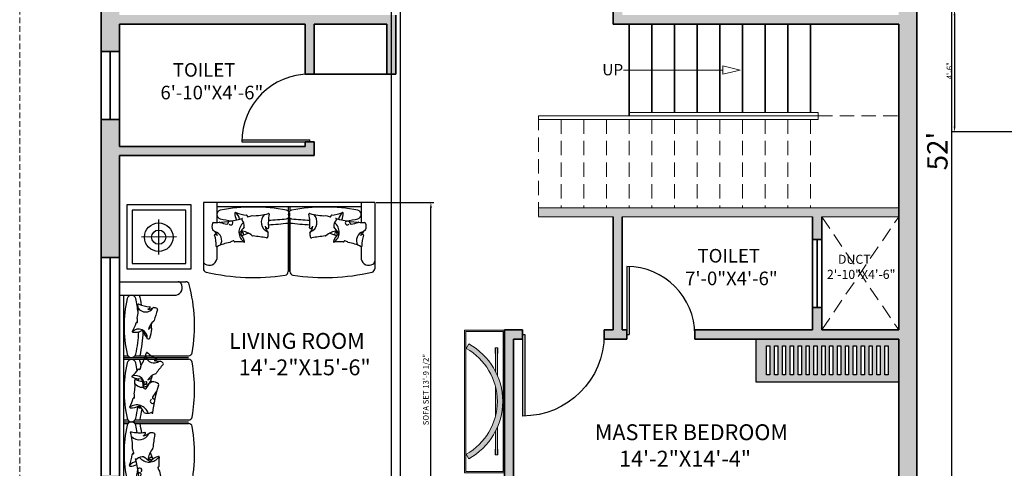
# Model space of a CAD drawing. Units: inches. Extents: x 1566 to 2546, y 1087 to 2705.
# Tile 6 of 27: x 1606 to 2040, y 1326 to 1524. Entities that reach past the tile are written whole.
import ezdxf

# ---------------------------------------------------------------- set-up
doc = ezdxf.new("R2010")
doc.units = ezdxf.units.IN
doc.linetypes.add('DASHED', pattern=[19.05, 12.7, -6.35])
for name, color, linetype, lineweight in [('A-ANNO-DIMS', 2, 'Continuous', 18), ('A-ANNO-TEXT', 7, 'Continuous', 18), ('A-AREA-IDEN', 7, 'Continuous', 18), ('A-DOOR', 4, 'Continuous', 25), ('A-FLOR-OVHD', 8, 'DASHED', 18), ('A-FLOR-STRS', 3, 'Continuous', 18), ('A-FURN', 8, 'Continuous', 18), ('A-WALL', 7, 'Continuous', 35), ('A-WALL-PATT', 8, 'Continuous', 13), ('aparador', 36, 'Continuous', 9), ('moveis', 254, 'Continuous', 5)]:
    doc.layers.add(name, color=color, linetype=linetype, lineweight=lineweight)
for name, color, linetype in [('HID', 11, 'Continuous'), ('MESA', 7, 'Continuous'), ('SAN', 5, 'Continuous'), ('wood', 26, 'Continuous')]:
    doc.layers.add(name, color=color, linetype=linetype)
doc.styles.get("Standard").update_dxf_attribs({"font": 'arial.ttf'})
doc.dimstyles.new('ISO-25', dxfattribs={"dimtxt": 2.5, "dimasz": 2.5, "dimexe": 1.25, "dimexo": 0.625, "dimtad": 1, "dimtxsty": 'Standard', "dimcen": 2.5, "dimadec": 0, "dimazin": 0, "dimtfac": 1, "dimtmove": 0, "dimatfit": 3, "dimfxl": 1, "dimarcsym": 0})

# ---------------------------------------------------------------- blocks, each defined once
blk = doc.blocks.new('d2')
for p, q in [((3364.08, 1632.29), (3364.08, 1602.29)), ((3365.08, 1632.29), (3365.08, 1602.29)), ((3364.08, 1602.29), (3365.08, 1602.29))]:
    blk.add_line(p, q)
at = {"ltscale": 0.3}
blk.add_arc((3364.08, 1602.29), 30, 0, 90, dxfattribs=at)
blk = doc.blocks.new('d1')
for p, q in [((3297.32, 1596.93), (3297.32, 1632.93)), ((3298.32, 1596.93), (3298.32, 1632.93)), ((3297.32, 1596.93), (3298.32, 1596.93))]:
    blk.add_line(p, q)
at = {"ltscale": 0.3}
blk.add_arc((3297.32, 1596.93), 36, 0, 90, dxfattribs=at)
blk = doc.blocks.new('*D7')
at = {"layer": 'A-ANNO-DIMS', "color": 0, "lineweight": -2, "transparency": 16777216}
for p, q in [((2002.15, 1778.2), (2018.24, 1778.2)), ((2016.99, 1156.7), (2016.99, 1775.7)), ((2002.15, 1154.2), (2018.24, 1154.2))]:
    blk.add_line(p, q, dxfattribs=at)
at = {"layer": 'A-ANNO-DIMS', "color": 0, "transparency": 16777216}
for points in [[(2016.58, 1775.7), (2017.41, 1775.7), (2016.99, 1778.2)], [(2016.58, 1156.7), (2017.41, 1156.7), (2016.99, 1154.2)]]:
    blk.add_solid(points, dxfattribs=at)
at = {"layer": 'Defpoints', "color": 0, "transparency": 16777216}
for p in [(2001.53, 1778.2), (2016.99, 1778.2), (2001.53, 1154.2)]:
    blk.add_point(p, dxfattribs=at)
at = {"layer": 'A-ANNO-DIMS', "color": 0, "transparency": 16777216, "insert": (2011.77, 1466.2), "char_height": 9, "attachment_point": 5, "rotation": 90}
blk.add_mtext("52'", dxfattribs=at)
blk = doc.blocks.new('Banco Lintz')
at = {"layer": 'MESA', "ltscale": 0.05}
h = blk.add_hatch(color=256, dxfattribs=at)
h.dxf.hatch_style = 1
h.set_gradient(color1=(138, 84, 66), color2=(0, 0, 0), one_color=1, name='INVCYLINDER')
h.paths.add_polyline_path([(0.48, 0), (0, 0), (0, -1.6), (0.48, -1.6)])
h.paths.add_polyline_path([(0.403, -0.509), (0.077, -0.509), (0.077, -0.472), (0.403, -0.472)], flags=16)
h.paths.add_polyline_path([(0.403, -0.561), (0.403, -0.597), (0.077, -0.597), (0.077, -0.561)], flags=16)
h.paths.add_polyline_path([(0.403, -0.421), (0.077, -0.421), (0.077, -0.384), (0.403, -0.384)], flags=16)
h.paths.add_polyline_path([(0.403, -0.649), (0.403, -0.686), (0.077, -0.686), (0.077, -0.649)], flags=16)
h.paths.add_polyline_path([(0.403, -0.332), (0.077, -0.332), (0.077, -0.296), (0.403, -0.296)], flags=16)
h.paths.add_polyline_path([(0.403, -0.737), (0.403, -0.774), (0.077, -0.774), (0.077, -0.737)], flags=16)
h.paths.add_polyline_path([(0.403, -0.244), (0.077, -0.244), (0.077, -0.207), (0.403, -0.207)], flags=16)
h.paths.add_polyline_path([(0.403, -0.826), (0.403, -0.863), (0.077, -0.863), (0.077, -0.826)], flags=16)
h.paths.add_polyline_path([(0.403, -0.156), (0.077, -0.156), (0.077, -0.119), (0.403, -0.119)], flags=16)
h.paths.add_polyline_path([(0.403, -0.914), (0.403, -0.951), (0.077, -0.951), (0.077, -0.914)], flags=16)
h.paths.add_polyline_path([(0.403, -1.003), (0.403, -1.039), (0.077, -1.039), (0.077, -1.003)], flags=16)
h.paths.add_polyline_path([(0.403, -1.091), (0.403, -1.128), (0.077, -1.128), (0.077, -1.091)], flags=16)
h.paths.add_polyline_path([(0.403, -1.179), (0.403, -1.216), (0.077, -1.216), (0.077, -1.179)], flags=16)
h.paths.add_polyline_path([(0.403, -1.268), (0.403, -1.304), (0.077, -1.304), (0.077, -1.268)], flags=16)
h.paths.add_polyline_path([(0.403, -1.356), (0.403, -1.393), (0.077, -1.393), (0.077, -1.356)], flags=16)
h.paths.add_polyline_path([(0.403, -1.444), (0.403, -1.481), (0.077, -1.481), (0.077, -1.444)], flags=16)
for points in [[(0, -1.6), (0.48, -1.6), (0.48, 0), (0, 0)], [(0.077, -0.119), (0.403, -0.119), (0.403, -0.156), (0.077, -0.156)], [(0.077, -0.207), (0.403, -0.207), (0.403, -0.244), (0.077, -0.244)], [(0.077, -0.296), (0.403, -0.296), (0.403, -0.332), (0.077, -0.332)], [(0.077, -0.384), (0.403, -0.384), (0.403, -0.421), (0.077, -0.421)], [(0.077, -0.472), (0.403, -0.472), (0.403, -0.509), (0.077, -0.509)], [(0.077, -0.561), (0.403, -0.561), (0.403, -0.597), (0.077, -0.597)], [(0.077, -0.649), (0.403, -0.649), (0.403, -0.686), (0.077, -0.686)], [(0.077, -0.737), (0.403, -0.737), (0.403, -0.774), (0.077, -0.774)], [(0.077, -0.826), (0.403, -0.826), (0.403, -0.863), (0.077, -0.863)], [(0.077, -0.914), (0.403, -0.914), (0.403, -0.951), (0.077, -0.951)], [(0.077, -1.003), (0.403, -1.003), (0.403, -1.039), (0.077, -1.039)], [(0.077, -1.091), (0.403, -1.091), (0.403, -1.128), (0.077, -1.128)], [(0.077, -1.179), (0.403, -1.179), (0.403, -1.216), (0.077, -1.216)], [(0.077, -1.268), (0.403, -1.268), (0.403, -1.304), (0.077, -1.304)], [(0.077, -1.356), (0.403, -1.356), (0.403, -1.393), (0.077, -1.393)], [(0.077, -1.444), (0.403, -1.444), (0.403, -1.481), (0.077, -1.481)]]:
    blk.add_lwpolyline(points, close=True, dxfattribs=at)
blk = doc.blocks.new('Aparador ORGANICA Formatto')
at = {"layer": 'aparador', "ltscale": 0.3}
h = blk.add_hatch(color=256, dxfattribs=at)
h.dxf.hatch_style = 1
h.set_gradient(color1=(118, 213, 123), color2=(52, 168, 57), one_color=1, tint=0.43, name='INVCURVED')
h.paths.add_polyline_path([(0.8, 0.45), (-0.8, 0.45), (-0.8, 0), (0.8, 0)])
h.paths.add_polyline_path([(0.785, 0.435), (0.785, 0.015), (-0.785, 0.015), (-0.785, 0.435)], flags=16)
h.paths.add_polyline_path([(0.291, 0.37), (0.537, 0.37), (0.537, 0.376), (0.601, 0.376), (0.601, 0.37), (0.601, 0.35), (0.601, 0.344), (0.537, 0.344), (0.537, 0.35), (0.334, 0.35, -0.150336), (0.645, 0.049), (0.592, 0.02, 0.208852), (0.163, 0.35), (-0.163, 0.35, 0.208852), (-0.592, 0.02), (-0.645, 0.049, -0.150336), (-0.334, 0.35), (-0.537, 0.35), (-0.537, 0.344), (-0.601, 0.344), (-0.601, 0.35), (-0.601, 0.37), (-0.601, 0.376), (-0.537, 0.376), (-0.537, 0.37), (-0.291, 0.37, -0.206106)], flags=0)
h = blk.add_hatch(color=256, dxfattribs=at)
h.dxf.hatch_style = 1
h.set_gradient(color1=(135, 92, 69), color2=(0, 0, 0), one_color=1, name='INVCURVED')
h.paths.add_polyline_path([(-0.645, 0.049), (-0.592, 0.02, -0.590888), (0.592, 0.02), (0.645, 0.049, 0.590888)])
h = blk.add_hatch(color=256, dxfattribs=at)
h.dxf.hatch_style = 1
h.set_gradient(color1=(178, 189, 189), one_color=1, tint=1, name='CYLINDER')
h.paths.add_polyline_path([(-0.537, 0.376), (-0.601, 0.376), (-0.601, 0.37), (-0.537, 0.37)])
h.paths.add_polyline_path([(-0.537, 0.35), (-0.601, 0.35), (-0.601, 0.344), (-0.537, 0.344)])
h = blk.add_hatch(color=256, dxfattribs=at)
h.dxf.hatch_style = 1
h.set_gradient(color1=(118, 213, 123), color2=(31, 101, 35), one_color=1, tint=0.26, name='INVCURVED')
h.paths.add_polyline_path([(-0.291, 0.37), (-0.601, 0.37), (-0.601, 0.35), (-0.334, 0.35, -0.015999)])
h = blk.add_hatch(color=256, dxfattribs=at)
h.dxf.hatch_style = 1
h.set_gradient(color1=(118, 213, 123), color2=(31, 101, 35), one_color=1, tint=0.26, name='INVCURVED')
h.paths.add_polyline_path([(-0.163, 0.35), (0.163, 0.35, 0.122516)])
h = blk.add_hatch(color=256, dxfattribs=at)
h.dxf.hatch_style = 1
h.set_gradient(color1=(118, 213, 123), color2=(31, 101, 35), one_color=1, tint=0.26, name='INVCURVED')
h.paths.add_polyline_path([(0.601, 0.37), (0.291, 0.37, -0.015999), (0.334, 0.35), (0.601, 0.35)])
h = blk.add_hatch(color=256, dxfattribs=at)
h.dxf.hatch_style = 1
h.set_gradient(color1=(178, 189, 189), one_color=1, tint=1, name='CYLINDER')
h.paths.add_polyline_path([(0.601, 0.376), (0.537, 0.376), (0.537, 0.37), (0.601, 0.37)])
h.paths.add_polyline_path([(0.601, 0.35), (0.537, 0.35), (0.537, 0.344), (0.601, 0.344)])
for p, q in [((-0.592, 0.02), (-0.645, 0.049)), ((0.592, 0.02), (0.645, 0.049))]:
    blk.add_line(p, q, dxfattribs=at)
for points in [[(-0.601, 0.37), (-0.601, 0.376), (-0.537, 0.376), (-0.537, 0.37)], [(-0.537, 0.35), (-0.537, 0.344), (-0.601, 0.344), (-0.601, 0.35)], [(0.601, 0.37), (0.601, 0.376), (0.537, 0.376), (0.537, 0.37)], [(0.537, 0.35), (0.537, 0.344), (0.601, 0.344), (0.601, 0.35)]]:
    blk.add_lwpolyline(points, dxfattribs=at)
for radius in [0.736, 0.676]:
    blk.add_arc((0, -0.306), radius, 28.8434, 151.1566, dxfattribs=at)
at = {"layer": 'moveis', "ltscale": 0.3}
for p, q in [((-0.601, 0.37), (-0.601, 0.35)), ((-0.291, 0.37), (-0.601, 0.37)), ((-0.601, 0.35), (-0.334, 0.35)), ((-0.163, 0.35), (0.163, 0.35)), ((0.291, 0.37), (0.601, 0.37)), ((0.601, 0.35), (0.334, 0.35)), ((0.601, 0.37), (0.601, 0.35))]:
    blk.add_line(p, q, dxfattribs=at)
for points in [[(-0.8, 0), (0.8, 0), (0.8, 0.45), (-0.8, 0.45)], [(-0.785, 0.015), (0.785, 0.015), (0.785, 0.435), (-0.785, 0.435)]]:
    blk.add_lwpolyline(points, close=True, dxfattribs=at)
blk = doc.blocks.new('123')
at = {"layer": 'HID'}
for centre, radius, start, end in [((1246.02, 1434.08), 0.283, 70.5302, 181.6176), ((1243.23, 1430.56), 4.68, 10.8696, 54.3073), ((1254.03, 1456.71), 23.73, 250.5302, 262.522), ((1285.34, 1456.71), 23.73, 277.478, 289.4698), ((1296.13, 1430.56), 4.68, 125.6927, 169.1304), ((1293.34, 1434.08), 0.283, 358.3824, 109.4698), ((1236.34, 1429.49), 0.472, 90.5535, 158.334), ((1235.86, 1479.09), 49.13, 270.5535, 285.4148), ((1235.86, 1479.09), 49.13, 270.5535, 273.614), ((1238.99, 1429.59), 0.472, 66.2045, 93.614), ((1245.71, 1450.89), 21.87, 252.6177, 260.951), ((1243.86, 1429.85), 1.05, 142.8444, 177.2985), ((1243.29, 1429.88), 0.472, 177.2985, 187.3574), ((1243.92, 1429.87), 0.999, 224.2238, 57.6435), ((1253.29, 1434.28), 7.55, 181.6176, 204.8398), ((1252.86, 1425.7), 5.32, 127.6048, 236.1053), ((1249.25, 1431.33), 0.472, 105.6578, 222.8337), ((1246.1, 1428.4), 3.83, 354.2387, 42.8337), ((1250.9, 1432.91), 0.283, 348.0525, 82.522), ((1251.46, 1432.79), 0.283, 168.0525, 279.4331), ((1249.65, 1443.68), 11.32, 279.4331, 289.3248), ((1254.03, 1456.71), 23.73, 268.4714, 286.0168), ((1262.09, 1430.12), 4.71, 134.8494, 245.9788), ((1279.38, 1429.58), 18.88, 167.7826, 186.0053), ((1260.65, 1433.64), 0.283, 347.7826, 106.0168), ((1278.71, 1433.64), 0.283, 73.9832, 192.2174), ((1259.98, 1429.58), 18.88, 353.9947, 12.2174), ((1285.34, 1456.71), 23.73, 253.9832, 271.5286), ((1277.28, 1430.12), 4.71, 294.0212, 45.1506), ((1289.72, 1443.68), 11.32, 250.6752, 260.5669), ((1287.91, 1432.79), 0.283, 260.5669, 11.9475), ((1288.46, 1432.91), 0.283, 97.478, 191.9475), ((1293.27, 1428.4), 3.83, 137.1663, 185.7613), ((1286.5, 1425.7), 5.32, 303.8947, 52.3952), ((1290.11, 1431.33), 0.472, 317.1663, 74.3422), ((1303.5, 1479.09), 49.13, 254.5852, 269.4465), ((1286.07, 1434.28), 7.55, 335.1602, 358.3824), ((1295.45, 1429.87), 0.999, 122.3565, 315.7762), ((1295.5, 1429.85), 1.05, 2.7015, 37.1556), ((1296.08, 1429.88), 0.472, 352.6426, 2.7015), ((1293.65, 1450.89), 21.87, 279.049, 287.3823), ((1300.38, 1429.59), 0.472, 86.386, 113.7955), ((1303.5, 1479.09), 49.13, 266.386, 269.4465), ((1303.02, 1429.49), 0.472, 21.666, 89.4465), ((1239.48, 1428.24), 3.85, 158.334, 202.6623), ((1236.36, 1426.94), 0.472, 202.6623, 238.3929), ((1233.54, 1422.36), 4.91, 20.2155, 58.3929), ((1236.02, 1422.11), 3.93, 326.1078, 77.2372), ((1242.35, 1429.76), 0.472, 260.951, 7.3574), ((1285.54, 1398.1), 46.53, 139.9755, 144.1671), ((1247.81, 1425.22), 0.945, 310.8427, 57.338), ((1253.61, 1432.21), 7.94, 229.38, 238.0577), ((1248.02, 1418.03), 8.16, 48.6039, 87.0681), ((1260.85, 1429.07), 1.87, 202.9525, 250.443), ((1264.95, 1429.26), 5.89, 188.9571, 220.4913), ((1260.32, 1427.58), 0.283, 250.443, 6.0053), ((1279.04, 1427.58), 0.283, 173.9947, 289.557), ((1274.42, 1429.26), 5.89, 319.5087, 351.0429), ((1278.51, 1429.07), 1.87, 289.557, 337.0475), ((1291.34, 1418.03), 8.16, 92.9319, 131.3961), ((1253.83, 1398.1), 46.53, 35.8329, 40.0245), ((1285.75, 1432.21), 7.94, 301.9423, 310.62), ((1291.56, 1425.22), 0.945, 122.662, 229.1573), ((1297.02, 1429.76), 0.472, 172.6426, 279.049), ((1303.34, 1422.11), 3.93, 102.7628, 213.8922), ((1305.82, 1422.36), 4.91, 121.6071, 159.7845), ((1303, 1426.94), 0.472, 301.6071, 337.3377), ((1299.88, 1428.24), 3.85, 337.3377, 21.666), ((1237.05, 1424.48), 0.236, 81.7015, 197.2637), ((1221.8, 1419.74), 15.74, 359.041, 17.2637), ((1236.86, 1423.18), 1.56, 34.2109, 81.7015), ((1248.4, 1413.06), 9.43, 110.6915, 120.5832), ((1245.15, 1421.66), 0.236, 359.311, 110.6915), ((1245.62, 1421.66), 0.236, 179.311, 273.7804), ((1246.94, 1401.69), 19.77, 81.7886, 93.7804), ((1248.01, 1425.2), 0.236, 144.1671, 251.1685), ((1243.89, 1420.15), 6.29, 12.876, 50.0789), ((1227.67, 1473.6), 52.85, 292.7112, 293.5018), ((1268.16, 1374.24), 53.54, 107.709, 111.2519), ((1248.79, 1424.95), 0.814, 313.9174, 40.1627), ((1249.8, 1421.5), 0.236, 261.7886, 12.876), ((1249.8, 1421.5), 0.236, 261.7886, 12.876), ((1253.8, 1424.57), 0.567, 227.5655, 264.8479), ((1248.46, 1365.29), 58.96, 79.0518, 84.8479), ((1259.76, 1423.73), 0.567, 259.0518, 342.8696), ((1256.05, 1424.88), 4.45, 342.8696, 7.2038), ((1283.31, 1424.88), 4.45, 172.7962, 197.1304), ((1279.6, 1423.73), 0.567, 197.1304, 280.9482), ((1290.9, 1365.29), 58.96, 95.1521, 100.9482), ((1285.56, 1424.57), 0.567, 275.1521, 312.4345), ((1271.2, 1374.24), 53.54, 68.7481, 72.291), ((1289.57, 1421.5), 0.236, 167.124, 278.2114), ((1289.57, 1421.5), 0.236, 167.124, 278.2114), ((1295.47, 1420.15), 6.29, 129.9211, 167.124), ((1292.43, 1401.69), 19.77, 86.2196, 98.2114), ((1290.58, 1424.95), 0.814, 139.8373, 226.0826), ((1311.69, 1473.6), 52.85, 246.4982, 247.2888), ((1291.36, 1425.2), 0.236, 288.8315, 35.8329), ((1293.75, 1421.66), 0.236, 266.2196, 0.689), ((1294.22, 1421.66), 0.236, 69.3085, 180.689), ((1290.97, 1413.06), 9.43, 59.4168, 69.3085), ((1302.5, 1423.18), 1.56, 98.2985, 145.7891), ((1317.56, 1419.74), 15.74, 162.7363, 180.959), ((1302.31, 1424.48), 0.236, 342.7363, 98.2985), ((1237.77, 1419.48), 0.236, 179.041, 297.2752), ((1246.94, 1401.69), 19.77, 99.7298, 117.2752), ((1292.43, 1401.69), 19.77, 62.7248, 80.2702), ((1301.6, 1419.48), 0.236, 242.7248, 0.959), ((1183.3, 1391.63), 19.77, 348.4714, 6.0168), ((1203.2, 1393.73), 0.236, 67.7826, 186.0168), ((1206.29, 1394.4), 3.93, 214.8494, 325.9788), ((1209.24, 1408.51), 15.74, 247.7826, 266.0053), ((1206.97, 1393.23), 1.56, 282.9525, 330.443), ((1207.41, 1396.62), 4.91, 268.9571, 300.4913), ((1208.12, 1392.58), 0.236, 330.443, 86.0053), ((1209.72, 1388.68), 3.71, 62.8696, 87.2038), ((1257.53, 1373.83), 49.13, 159.0518, 164.8479), ((1211.2, 1391.57), 0.472, 339.0518, 62.8696), ((1193.36, 1386.15), 9.43, 359.4331, 9.3248), ((1209.64, 1386.8), 0.472, 307.5655, 344.8479), ((1203.21, 1378.98), 3.9, 356.4825, 134.3073), ((1183.3, 1391.63), 19.77, 330.5302, 342.522), ((1201.6, 1387.78), 6.29, 261.6176, 299.5758), ((1202.38, 1385.62), 0.236, 68.0525, 162.522), ((1202.56, 1386.06), 0.236, 248.0525, 359.4331), ((1204.83, 1382.1), 0.236, 32.8897, 119.5758), ((1165.95, 1356.96), 46.53, 28.8632, 32.8897), ((1213.67, 1381.56), 6.13, 127.5655, 169.079), ((1204.32, 1386.81), 5.27, 309.1869, 318.5341), ((1191.35, 1384.83), 17.84, 340.6607, 353.8744), ((1208.63, 1383.01), 0.472, 349.5475, 138.5341), ((1199.58, 1383.44), 9.43, 359.0692, 11.4619), ((1200.72, 1381.79), 0.236, 150.5302, 261.6176), ((1207.62, 1379.5), 0.917, 184.9476, 286.1991), ((1207.74, 1379.07), 0.472, 286.1991, 340.6607), ((1187.51, 1377.19), 19.77, 328.4714, 346.0168), ((1210.06, 1371.93), 3.93, 194.8494, 305.9788), ((1206.93, 1372.36), 0.236, 47.7826, 166.0168), ((1217.66, 1384.18), 15.74, 227.7826, 246.0053), ((1210.31, 1370.6), 1.56, 262.9525, 310.443), ((1211.88, 1373.63), 4.91, 248.9571, 280.4913), ((1211.17, 1369.59), 0.236, 310.443, 66.0053), ((1187.51, 1377.19), 19.77, 310.5302, 322.522), ((1203.39, 1365.02), 0.236, 48.0525, 142.522), ((1203.71, 1365.37), 0.236, 228.0525, 339.4331), ((1195.1, 1368.6), 9.43, 339.4331, 349.3248), ((1251.18, 1335.08), 49.13, 139.0518, 144.8479), ((1211.34, 1365.39), 3.71, 42.8696, 67.2038), ((1213.71, 1367.59), 0.472, 319.0518, 42.8696), ((1200.52, 1361.98), 0.236, 130.5302, 241.6176), ((1201.9, 1358.5), 3.9, 336.4825, 114.3073), ((1203.4, 1367.31), 6.29, 241.6176, 279.5758), ((1181.91, 1357.9), 19.77, 349.7298, 7.2752), ((1201.76, 1360.43), 0.236, 69.041, 187.2752), ((1207.47, 1375.34), 15.74, 249.041, 267.2637), ((1204.48, 1360.87), 0.236, 12.8897, 99.5758), ((1159.36, 1350.55), 46.53, 8.8632, 12.8897), ((1212.61, 1357.35), 6.13, 107.5655, 149.079), ((1205.62, 1365.47), 5.27, 289.1869, 298.5341), ((1208.36, 1360.43), 0.472, 329.5475, 118.5341), ((1200.01, 1363.93), 9.43, 339.0692, 351.4619), ((1210.62, 1363.64), 0.472, 287.5655, 324.8479), ((1204.83, 1361.17), 3.93, 216.1078, 327.2372), ((1206.22, 1357.48), 0.917, 164.9476, 266.1991), ((1205.91, 1363.41), 4.91, 270.2155, 308.3929), ((1205.54, 1360.02), 1.56, 284.2109, 331.7015), ((1206.19, 1357.03), 0.472, 266.1991, 320.6607), ((1192.75, 1368.04), 17.84, 320.6607, 333.8744), ((1206.71, 1359.39), 0.236, 331.7015, 87.2637), ((1209.25, 1359.2), 0.472, 92.6623, 128.3929), ((1209.41, 1355.82), 3.85, 48.334, 92.6623), ((1258.43, 1341.83), 49.13, 160.5535, 175.4148), ((1258.43, 1341.83), 49.13, 160.5535, 163.614), ((1211.66, 1358.35), 0.472, 340.5535, 48.334), ((1181.91, 1357.9), 19.77, 331.7886, 343.7804), ((1201.12, 1352.31), 0.236, 69.311, 163.7804), ((1201.29, 1352.75), 0.236, 249.311, 0.6915), ((1192.09, 1352.64), 9.43, 0.6915, 10.5832), ((1209.42, 1351.1), 0.999, 114.2238, 307.6435), ((1209.85, 1352.61), 0.472, 150.951, 257.3574), ((1228.56, 1342.22), 21.87, 142.6177, 150.951), ((1209.65, 1351.69), 0.472, 67.2985, 77.3574), ((1209.42, 1351.16), 1.05, 32.8444, 67.2985), ((1210.84, 1355.82), 0.472, 316.2045, 343.614), ((1202.44, 1344.12), 5.32, 17.6048, 126.1053), ((1199.54, 1348.44), 0.236, 151.7886, 262.876), ((1199.54, 1348.44), 0.236, 151.7886, 262.876), ((1200.29, 1354.45), 6.29, 262.876, 300.0789), ((1203.73, 1349.03), 0.945, 200.8427, 307.338), ((1256.07, 1351.41), 52.85, 182.7112, 183.5018), ((1203.63, 1348.85), 0.236, 34.1671, 141.1685), ((1165.33, 1322.86), 46.53, 29.9755, 34.1671), ((1155.85, 1369.08), 52.85, 337.2794, 337.2982), ((1207.3, 1349.55), 3.83, 244.2387, 292.8337), ((1208.97, 1345.59), 0.472, 355.6578, 112.8337), ((1199.97, 1337.3), 0.283, 77.7826, 196.0168), ((1176.89, 1330.67), 23.73, 358.4714, 16.0168), ((1204.03, 1356.03), 18.88, 257.7826, 276.0053), ((1203.48, 1338.74), 4.71, 224.8494, 335.9788), ((1204.35, 1341.6), 5.89, 278.9571, 310.4913), ((1204.54, 1337.5), 1.87, 292.9525, 340.443), ((1206.03, 1336.97), 0.283, 340.443, 96.0053), ((1208.73, 1332.7), 4.45, 72.8696, 97.2038), ((1268.32, 1325.11), 58.96, 169.0518, 174.8479), ((1209.88, 1336.41), 0.567, 349.0518, 72.8696), ((1189.93, 1326.3), 11.32, 9.4331, 19.3248), ((1215.58, 1324.67), 8.16, 138.6039, 177.0681), ((1209.03, 1330.45), 0.567, 317.5655, 354.8479), ((1176.89, 1330.67), 23.73, 340.5302, 352.522), ((1200.7, 1327.55), 0.283, 78.0525, 172.522), ((1200.82, 1328.1), 0.283, 258.0525, 9.4331), ((1202.28, 1325.9), 0.472, 195.6578, 312.8337), ((1205.2, 1322.75), 3.83, 84.2387, 132.8337), ((1207.91, 1329.51), 5.32, 217.6048, 326.1053), ((1235.51, 1362.19), 46.53, 229.9755, 234.1671), ((1201.4, 1330.26), 7.94, 319.38, 328.0577), ((1208.66, 1325.44), 0.814, 43.9174, 130.1627), ((1259.37, 1344.81), 53.54, 197.709, 201.2519), ((1213.46, 1320.54), 6.29, 102.876, 140.0789), ((1212.11, 1326.45), 0.236, 351.7886, 102.876), ((1212.11, 1326.45), 0.236, 351.7886, 102.876), ((1231.92, 1323.59), 19.77, 171.7886, 183.7804), ((1203.05, 1319.88), 4.68, 100.8696, 144.3073), ((1199.53, 1322.67), 0.283, 160.5302, 271.6176), ((1199.33, 1329.94), 7.55, 271.6176, 294.8398), ((1154.52, 1312.51), 49.13, 0.5535, 15.4148), ((1203.74, 1320.57), 0.999, 314.2238, 147.6435), ((1208.38, 1324.46), 0.945, 40.8427, 147.338), ((1208.41, 1324.65), 0.236, 234.1671, 341.1685), ((1160.01, 1304.32), 52.85, 22.7112, 23.5018), ((1211.95, 1321.8), 0.236, 89.311, 200.6915), ((1220.55, 1325.05), 9.43, 200.6915, 210.5832), ((1211.95, 1322.27), 0.236, 269.311, 3.7804), ((1203.76, 1320.51), 1.05, 232.8444, 267.2985), ((1182.72, 1322.36), 21.87, 342.6177, 350.951), ((1203.73, 1319.94), 0.472, 267.2985, 277.3574), ((1203.85, 1319), 0.472, 350.951, 97.3574), ((1231.92, 1323.59), 19.77, 189.7298, 207.2752), ((1204.02, 1315.64), 0.472, 156.2045, 183.614), ((1154.52, 1312.51), 49.13, 0.5535, 3.614), ((1204.12, 1312.99), 0.472, 180.5535, 248.334), ((1205.37, 1316.13), 3.85, 248.334, 292.6623), ((1206.67, 1313.01), 0.472, 292.6623, 328.3929), ((1211.25, 1310.19), 4.91, 110.2155, 148.3929), ((1211.49, 1312.67), 3.93, 56.1078, 167.2372), ((1210.43, 1313.51), 1.56, 124.2109, 171.7015), ((1209.12, 1313.7), 0.236, 171.7015, 287.2637), ((1213.86, 1298.45), 15.74, 89.041, 107.2637), ((1214.13, 1314.42), 0.236, 269.041, 27.2752), ((1221.8, 1292.6), 15.74, 342.7363, 0.959), ((1236.02, 1290.24), 3.93, 282.7628, 33.8922), ((1237.77, 1292.87), 0.236, 62.7248, 180.959), ((1246.94, 1310.66), 19.77, 242.7248, 260.2702), ((1248.4, 1299.29), 9.43, 239.4168, 249.3085), ((1245.62, 1290.69), 0.236, 86.2196, 180.689), ((1246.94, 1310.66), 19.77, 266.2196, 278.2114), ((1252.86, 1286.65), 5.32, 123.8947, 232.3952), ((1249.8, 1290.85), 0.236, 347.124, 98.2114), ((1249.8, 1290.85), 0.236, 347.124, 98.2114), ((1289.57, 1290.85), 0.236, 81.7886, 192.876), ((1289.57, 1290.85), 0.236, 81.7886, 192.876), ((1286.5, 1286.65), 5.32, 307.6048, 56.1053), ((1292.43, 1310.66), 19.77, 261.7886, 273.7804), ((1293.75, 1290.69), 0.236, 359.311, 93.7804), ((1290.97, 1299.29), 9.43, 290.6915, 300.5832), ((1292.43, 1310.66), 19.77, 279.7298, 297.2752), ((1303.34, 1290.24), 3.93, 146.1078, 257.2372), ((1301.6, 1292.87), 0.236, 359.041, 117.2752), ((1317.56, 1292.6), 15.74, 179.041, 197.2637), ((1233.54, 1289.99), 4.91, 301.6071, 339.7845), ((1237.05, 1287.87), 0.236, 162.7363, 278.2985), ((1236.86, 1289.17), 1.56, 278.2985, 325.7891), ((1245.15, 1290.69), 0.236, 249.3085, 0.689), ((1248.01, 1287.15), 0.236, 108.8315, 215.8329), ((1285.54, 1314.25), 46.53, 215.8329, 220.0245), ((1243.89, 1292.2), 6.29, 309.9211, 347.124), ((1227.67, 1238.75), 52.85, 66.4982, 67.2888), ((1247.81, 1287.12), 0.945, 302.662, 49.1573), ((1248.02, 1294.32), 8.16, 272.9319, 311.3961), ((1253.61, 1280.14), 7.94, 121.9423, 130.62), ((1268.16, 1338.11), 53.54, 248.7481, 252.291), ((1248.79, 1287.4), 0.814, 319.8373, 46.0826), ((1253.8, 1287.77), 0.567, 95.1521, 132.4345), ((1248.46, 1347.06), 58.96, 275.1521, 280.9482), ((1262.09, 1282.22), 4.71, 114.0212, 225.1506), ((1264.95, 1283.09), 5.89, 139.5087, 171.0429), ((1259.76, 1288.62), 0.567, 17.1304, 100.9482), ((1256.05, 1287.47), 4.45, 352.7962, 17.1304), ((1283.31, 1287.47), 4.45, 162.8696, 187.2038), ((1274.42, 1283.09), 5.89, 8.9571, 40.4913), ((1279.6, 1288.62), 0.567, 79.0518, 162.8696), ((1277.28, 1282.22), 4.71, 314.8494, 65.9788), ((1290.9, 1347.06), 58.96, 259.0518, 264.8479), ((1285.56, 1287.77), 0.567, 47.5655, 84.8479), ((1291.34, 1294.32), 8.16, 228.6039, 267.0681), ((1271.2, 1338.11), 53.54, 287.709, 291.2519), ((1295.47, 1292.2), 6.29, 192.876, 230.0789), ((1253.83, 1314.25), 46.53, 319.9755, 324.1671), ((1290.58, 1287.4), 0.814, 133.9174, 220.1627), ((1285.75, 1280.14), 7.94, 49.38, 58.0577), ((1291.56, 1287.12), 0.945, 130.8427, 237.338), ((1311.69, 1238.75), 52.85, 112.7112, 113.5018), ((1291.36, 1287.15), 0.236, 324.1671, 71.1685), ((1294.22, 1290.69), 0.236, 179.311, 290.6915), ((1302.5, 1289.17), 1.56, 214.2109, 261.7015), ((1305.82, 1289.99), 4.91, 200.2155, 238.3929), ((1302.31, 1287.87), 0.236, 261.7015, 17.2637), ((1239.48, 1284.11), 3.85, 157.3377, 201.666), ((1236.34, 1282.86), 0.472, 201.666, 269.4465), ((1236.36, 1285.41), 0.472, 121.6071, 157.3377), ((1235.86, 1233.26), 49.13, 74.5852, 89.4465), ((1235.86, 1233.26), 49.13, 86.386, 89.4465), ((1238.99, 1282.76), 0.472, 266.386, 293.7955), ((1245.71, 1261.46), 21.87, 99.049, 107.3823), ((1242.35, 1282.59), 0.472, 352.6426, 99.049), ((1243.29, 1282.47), 0.472, 172.6426, 182.7015), ((1243.86, 1282.5), 1.05, 182.7015, 217.1556), ((1243.92, 1282.48), 0.999, 302.3565, 135.7762), ((1246.1, 1283.94), 3.83, 317.1663, 5.7613), ((1260.85, 1283.28), 1.87, 109.557, 157.0475), ((1260.32, 1284.77), 0.283, 353.9947, 109.557), ((1279.38, 1282.77), 18.88, 173.9947, 192.2174), ((1259.98, 1282.77), 18.88, 347.7826, 6.0053), ((1279.04, 1284.77), 0.283, 70.443, 186.0053), ((1278.51, 1283.28), 1.87, 22.9525, 70.443), ((1293.27, 1283.94), 3.83, 174.2387, 222.8337), ((1303.5, 1233.26), 49.13, 90.5535, 105.4148), ((1295.45, 1282.48), 0.999, 44.2238, 237.6435), ((1295.5, 1282.5), 1.05, 322.8444, 357.2985), ((1297.02, 1282.59), 0.472, 80.951, 187.3574), ((1296.08, 1282.47), 0.472, 357.2985, 7.3574), ((1293.65, 1261.46), 21.87, 72.6177, 80.951), ((1300.38, 1282.76), 0.472, 246.2045, 273.614), ((1303.5, 1233.26), 49.13, 90.5535, 93.614), ((1303.02, 1282.86), 0.472, 270.5535, 338.334), ((1303, 1285.41), 0.472, 22.6623, 58.3929), ((1299.88, 1284.11), 3.85, 338.334, 22.6623), ((1253.29, 1278.07), 7.55, 155.1602, 178.3824), ((1246.02, 1278.27), 0.283, 178.3824, 289.4698), ((1243.23, 1281.79), 4.68, 305.6927, 349.1304), ((1254.03, 1255.63), 23.73, 97.478, 109.4698), ((1249.25, 1281.02), 0.472, 137.1663, 254.3422), ((1250.9, 1279.44), 0.283, 277.478, 11.9475), ((1251.46, 1279.56), 0.283, 80.5669, 191.9475), ((1249.65, 1268.67), 11.32, 70.6752, 80.5669), ((1254.03, 1255.63), 23.73, 73.9832, 91.5286), ((1260.65, 1278.71), 0.283, 253.9832, 12.2174), ((1278.71, 1278.71), 0.283, 167.7826, 286.0168), ((1285.34, 1255.63), 23.73, 88.4714, 106.0168), ((1289.72, 1268.67), 11.32, 99.4331, 109.3248), ((1287.91, 1279.56), 0.283, 348.0525, 99.4331), ((1288.46, 1279.44), 0.283, 168.0525, 262.522), ((1285.34, 1255.63), 23.73, 70.5302, 82.522), ((1290.11, 1281.02), 0.472, 285.6578, 42.8337), ((1296.13, 1281.79), 4.68, 190.8696, 234.3073), ((1286.07, 1278.07), 7.55, 1.6176, 24.8398), ((1293.34, 1278.27), 0.283, 250.5302, 1.6176)]:
    blk.add_arc(centre, radius, start, end, dxfattribs=at)
at = {"layer": 'SAN'}
for p, q in [((1212.06, 1431.34), (1212.06, 1415.9)), ((1220, 1423.66), (1204.47, 1423.49)), ((1212.06, 1281.01), (1212.06, 1296.45)), ((1220, 1288.69), (1204.47, 1288.86))]:
    blk.add_line(p, q, dxfattribs=at)
for centre, radius in [((1212.15, 1423.49), 6.3), ((1212.15, 1423.49), 3.15), ((1212.15, 1288.86), 6.3), ((1212.15, 1288.86), 3.15)]:
    blk.add_circle(centre, radius, dxfattribs=at)
at = {"layer": 'wood'}
for p, q in [((1307.48, 1438.84), (1231.89, 1438.84)), ((1231.89, 1438.84), (1231.89, 1409.55)), ((1237.79, 1438.84), (1237.79, 1430)), ((1301.57, 1438.84), (1301.57, 1430)), ((1307.48, 1438.84), (1307.48, 1409.55)), ((1301.57, 1436.87), (1237.79, 1436.87)), ((1269.29, 1436.87), (1269.29, 1435.11)), ((1270.08, 1436.87), (1270.08, 1435.11)), ((1269.29, 1431.89), (1269.29, 1408.27)), ((1269.68, 1431.89), (1269.68, 1408.27)), ((1270.08, 1431.89), (1270.08, 1408.27)), ((1237.79, 1419.24), (1237.79, 1413.76)), ((1301.57, 1419.24), (1301.57, 1413.76)), ((1194.77, 1308.54), (1194.77, 1403.81)), ((1194.77, 1403.81), (1224.06, 1403.81)), ((1194.77, 1397.91), (1219.85, 1397.91)), ((1196.74, 1314.44), (1196.74, 1397.91)), ((1196.74, 1371.13), (1198.49, 1371.13)), ((1196.74, 1370.35), (1225.34, 1370.35)), ((1196.74, 1369.56), (1225.34, 1369.56)), ((1201.72, 1371.13), (1225.34, 1371.13)), ((1196.74, 1342.79), (1198.49, 1342.79)), ((1196.74, 1342), (1225.34, 1342)), ((1196.74, 1341.21), (1198.49, 1341.21)), ((1201.72, 1342.79), (1225.34, 1342.79)), ((1201.72, 1341.21), (1225.34, 1341.21)), ((1194.77, 1314.44), (1203.61, 1314.44)), ((1214.37, 1314.44), (1219.85, 1314.44)), ((1194.77, 1308.54), (1224.06, 1308.54)), ((1269.29, 1280.46), (1269.29, 1304.08)), ((1269.68, 1280.46), (1269.68, 1304.08)), ((1270.08, 1280.46), (1270.08, 1304.08)), ((1231.89, 1273.51), (1231.89, 1302.8)), ((1307.48, 1273.51), (1307.48, 1302.8)), ((1237.79, 1293.11), (1237.79, 1298.59)), ((1301.57, 1293.11), (1301.57, 1298.59)), ((1237.79, 1273.51), (1237.79, 1282.35)), ((1301.57, 1273.51), (1301.57, 1282.35)), ((1307.48, 1273.51), (1231.89, 1273.51)), ((1301.57, 1275.48), (1237.79, 1275.48)), ((1269.29, 1275.48), (1269.29, 1277.24)), ((1270.08, 1275.48), (1270.08, 1277.24))]:
    blk.add_line(p, q, dxfattribs=at)
for points in [[(1198.13, 1409.44), (1226.48, 1409.44), (1226.48, 1437.78), (1198.13, 1437.78)], [(1200.49, 1411.8), (1224.11, 1411.8), (1224.11, 1435.42), (1200.49, 1435.42)], [(1198.13, 1302.91), (1226.48, 1302.91), (1226.48, 1274.57), (1198.13, 1274.57)], [(1200.49, 1300.55), (1224.11, 1300.55), (1224.11, 1276.93), (1200.49, 1276.93)]]:
    blk.add_lwpolyline(points, close=True, dxfattribs=at)
for centre, radius, start, end in [((1239.8, 1433.5), 1.97, 104.0803, 255.9197), ((1253.99, 1357.1), 79.67, 79.4658, 100.6108), ((1268.09, 1433.5), 1.98, 283.4421, 76.5579), ((1271.27, 1433.5), 1.98, 103.4421, 256.5579), ((1285.38, 1357.1), 79.67, 79.3892, 100.5342), ((1299.57, 1433.5), 1.97, 284.0803, 75.9197), ((1251.62, 1486.43), 56.2, 257.3591, 262.5789), ((1239.14, 1754.92), 324.68, 273.7815, 275.1985), ((1300.23, 1754.92), 324.68, 264.8015, 266.2185), ((1287.75, 1486.43), 56.2, 277.4211, 282.6409), ((1241.58, 1693.38), 265.11, 274.0948, 275.9995), ((1297.79, 1693.38), 265.11, 264.0005, 265.9052), ((1233.46, 1412.91), 1.57, 180, 238.6411), ((1234.43, 1414.5), 3.44, 238.6411, 347.5888), ((1304.93, 1414.5), 3.44, 192.4112, 301.3589), ((1305.9, 1412.91), 1.57, 301.3589, 0), ((1233.46, 1409.55), 1.57, 180, 255.2393), ((1267.71, 1408.27), 1.57, 279.7794, 0), ((1271.65, 1408.27), 1.57, 180, 260.2206), ((1305.9, 1409.55), 1.57, 284.7607, 0), ((1254.02, 1500.46), 94.78, 257.2232, 278.4687), ((1285.34, 1500.46), 94.78, 261.5313, 282.7768), ((1219.11, 1401.27), 3.44, 282.4112, 31.3589), ((1220.7, 1402.24), 1.57, 31.3589, 90), ((1224.06, 1402.24), 1.57, 14.7607, 90), ((1156.82, 1384.52), 71.11, 350.2206, 14.7607), ((1253.04, 1384.08), 56.2, 167.3591, 192.5496), ((1200.11, 1395.9), 1.97, 14.0803, 165.9197), ((1147.18, 1384.08), 56.2, 6.399, 12.6409), ((1147.18, 1384.08), 58.17, 9.2978, 13.7486), ((1147.18, 1384.08), 56.2, 347.4504, 357.5986), ((1147.18, 1384.08), 58.17, 347.1404, 357.743), ((1200.11, 1372.33), 1.98, 193.4421, 346.5579), ((1200.11, 1367.56), 1.97, 14.0803, 165.9197), ((1147.18, 1355.74), 58.17, 10.7847, 13.7486), ((1225.34, 1372.71), 1.57, 270, 350.2206), ((1225.34, 1367.99), 1.57, 9.7794, 90), ((1253.04, 1355.74), 56.2, 167.3591, 192.5496), ((1147.18, 1355.74), 56.2, 8.9885, 12.6409), ((1156.82, 1356.17), 71.11, 350.2206, 9.7794), ((1147.18, 1355.74), 56.2, 4.5548, 5.3997), ((1147.18, 1355.74), 56.2, 347.4504, 352.6454), ((1147.18, 1355.74), 58.17, 347.1404, 351.9048), ((1200.11, 1343.98), 1.98, 193.4421, 346.5579), ((1225.34, 1344.36), 1.57, 270, 350.2206), ((1253.04, 1328.27), 56.2, 167.4504, 192.6409), ((1200.11, 1340.02), 1.98, 13.4421, 166.5579), ((1147.18, 1328.27), 56.2, 9.1435, 12.5496), ((1147.18, 1328.27), 58.17, 8.7934, 12.8596), ((1225.34, 1339.64), 1.57, 9.7794, 90), ((1156.82, 1327.83), 71.11, 345.2393, 9.7794), ((1147.18, 1328.27), 56.2, 347.3591, 352.5789), ((1200.11, 1316.45), 1.97, 194.0803, 345.9197), ((1219.11, 1311.08), 3.44, 328.6411, 77.5888), ((1220.7, 1310.11), 1.57, 270, 328.6411), ((1224.06, 1310.11), 1.57, 270, 345.2393), ((1233.46, 1302.8), 1.57, 104.7607, 180), ((1254.02, 1211.88), 94.78, 81.5313, 102.7768), ((1267.71, 1304.08), 1.57, 0, 80.2206), ((1271.65, 1304.08), 1.57, 99.7794, 180), ((1285.34, 1211.88), 94.78, 77.2232, 98.4687), ((1305.9, 1302.8), 1.57, 0, 75.2393), ((1233.46, 1299.44), 1.57, 121.3589, 180), ((1234.43, 1297.85), 3.44, 12.4112, 121.3589), ((1304.93, 1297.85), 3.44, 58.6411, 167.5888), ((1305.9, 1299.44), 1.57, 0, 58.6411), ((1241.58, 1018.97), 265.11, 84.0005, 85.9052), ((1297.79, 1018.97), 265.11, 94.0948, 95.9995), ((1239.8, 1278.85), 1.97, 104.0803, 255.9197), ((1251.62, 1225.92), 56.2, 97.4211, 102.6409), ((1239.14, 957.43), 324.68, 84.8015, 86.2185), ((1268.09, 1278.85), 1.98, 283.4421, 76.5579), ((1271.27, 1278.85), 1.98, 103.4421, 256.5579), ((1300.23, 957.43), 324.68, 93.7815, 95.1985), ((1287.75, 1225.92), 56.2, 77.3591, 82.5789), ((1299.57, 1278.85), 1.97, 284.0803, 75.9197), ((1253.99, 1355.25), 79.67, 259.3892, 280.5342), ((1285.38, 1355.25), 79.67, 259.4658, 280.6108)]:
    blk.add_arc(centre, radius, start, end, dxfattribs=at)
blk = doc.blocks.new('*D61')
at = {"layer": 'A-ANNO-DIMS', "color": 0, "lineweight": -2, "transparency": 16777216}
for p, q in [((1762.86, 1443.53), (1788.29, 1443.53)), ((1787.04, 1280.7), (1787.04, 1441.03)), ((1762.86, 1278.2), (1788.29, 1278.2))]:
    blk.add_line(p, q, dxfattribs=at)
at = {"layer": 'A-ANNO-DIMS', "color": 0, "transparency": 16777216}
for points in [[(1786.62, 1441.03), (1787.46, 1441.03), (1787.04, 1443.53)], [(1786.62, 1280.7), (1787.46, 1280.7), (1787.04, 1278.2)]]:
    blk.add_solid(points, dxfattribs=at)
at = {"layer": 'Defpoints', "color": 0, "transparency": 16777216}
for p in [(1762.24, 1443.53), (1787.04, 1443.53), (1762.24, 1278.2)]:
    blk.add_point(p, dxfattribs=at)
at = {"layer": 'A-ANNO-DIMS', "color": 0, "transparency": 16777216, "insert": (1785.12, 1360.86), "char_height": 2.5, "attachment_point": 5, "rotation": 90}
blk.add_mtext('SOFA SET 13\'-9 1/2"', dxfattribs=at)
blk = doc.blocks.new('*D92')
at = {"layer": 'A-ANNO-DIMS', "color": 0, "lineweight": -2, "transparency": 16777216}
for p, q in [((2061.66, 1528.68), (2016.94, 1528.68)), ((2018.19, 1526.18), (2018.19, 1477.15)), ((2061.66, 1474.65), (2016.94, 1474.65))]:
    blk.add_line(p, q, dxfattribs=at)
at = {"layer": 'A-ANNO-DIMS', "color": 0, "transparency": 16777216}
for points in [[(2017.77, 1526.18), (2018.6, 1526.18), (2018.19, 1528.68)], [(2017.77, 1477.15), (2018.6, 1477.15), (2018.19, 1474.65)]]:
    blk.add_solid(points, dxfattribs=at)
at = {"layer": 'Defpoints', "color": 0, "transparency": 16777216}
for p in [(2062.29, 1528.68), (2018.19, 1474.65), (2062.29, 1474.65)]:
    blk.add_point(p, dxfattribs=at)
at = {"layer": 'A-ANNO-DIMS', "color": 0, "transparency": 16777216, "insert": (2016.29, 1501.66), "char_height": 2.5, "attachment_point": 5, "rotation": 90}
blk.add_mtext('4\'-6"', dxfattribs=at)
blk = doc.blocks.new('*D110')
at = {"layer": 'A-ANNO-DIMS', "color": 0, "lineweight": -2, "transparency": 16777216}
for p, q in [((1769.53, 1769.57), (1769.53, 1087.35)), ((1773.53, 1769.57), (1773.53, 1087.35)), ((1767.03, 1088.6), (1764.53, 1088.6)), ((1769.53, 1088.6), (1773.53, 1088.6)), ((1776.03, 1088.6), (1786.43, 1088.6))]:
    blk.add_line(p, q, dxfattribs=at)
at = {"layer": 'A-ANNO-DIMS', "color": 0, "transparency": 16777216}
for points in [[(1767.03, 1089.01), (1767.03, 1088.18), (1769.53, 1088.6)], [(1776.03, 1089.01), (1776.03, 1088.18), (1773.53, 1088.6)]]:
    blk.add_solid(points, dxfattribs=at)
at = {"layer": 'Defpoints', "color": 0, "transparency": 16777216}
for p in [(1769.53, 1770.2), (1773.53, 1770.2), (1773.53, 1088.6)]:
    blk.add_point(p, dxfattribs=at)
at = {"layer": 'A-ANNO-DIMS', "color": 0, "transparency": 16777216, "insert": (1782.48, 1090.5), "char_height": 2.5, "attachment_point": 5}
blk.add_mtext('0\'-4"', dxfattribs=at)

msp = doc.modelspace()

# ---------------------------------------------------------------- hatches: boundary and pattern name
at = {"layer": 'A-WALL-PATT'}
h = msp.add_hatch(color=256, dxfattribs=at)
h.dxf.hatch_style = 1
h.paths.add_polyline_path([(2001.53, 1778.2), (1641.53, 1778.2), (1641.53, 1746.2), (1649.53, 1746.2), (1649.53, 1770.2), (1769.53, 1770.2), (1769.53, 1650.2), (1767.53, 1650.2), (1767.53, 1648.2), (1767.53, 1646.2), (1819.53, 1646.2), (1819.53, 1650.2), (1773.53, 1650.2), (1773.53, 1770.2), (1941.53, 1770.2), (1941.53, 1756.2), (1945.53, 1756.2), (1945.53, 1770.2), (1993.53, 1770.2), (1993.53, 1650.2), (1945.53, 1650.2), (1945.53, 1652.2), (1943.53, 1652.2), (1941.53, 1652.2), (1941.53, 1650.2), (1867.53, 1650.2), (1867.53, 1642.2), (1871.53, 1642.2), (1871.53, 1646.2), (1993.53, 1646.2), (1993.53, 1526.2), (1871.53, 1526.2), (1871.53, 1606.2), (1867.53, 1606.2), (1867.53, 1522.2), (1993.53, 1522.2), (1993.53, 1387.2), (1959.53, 1387.2), (1959.53, 1397.2), (1955.53, 1397.2), (1955.53, 1387.2), (1903.53, 1387.2), (1903.53, 1383.2), (1993.53, 1383.2), (1993.53, 1364.3), (1993.53, 1211.2), (1939.53, 1211.2), (1939.53, 1203.2), (1993.53, 1203.2), (1993.53, 1154.2), (2001.53, 1154.2)])
h.paths.add_polyline_path([(1649.53, 1646.2), (1731.53, 1646.2), (1731.53, 1650.2), (1649.53, 1650.2), (1649.53, 1674.2), (1641.53, 1674.2), (1641.53, 1622.2), (1649.53, 1622.2)], flags=17)
h.paths.add_polyline_path([(1649.53, 1550.2), (1641.53, 1550.2), (1641.53, 1510.2), (1649.53, 1510.2), (1649.53, 1522.2), (1731.53, 1522.2), (1731.53, 1500.2), (1735.53, 1500.2), (1735.53, 1522.2), (1767.53, 1522.2), (1767.53, 1500.2), (1771.53, 1500.2), (1771.53, 1526.2), (1649.53, 1526.2)], flags=17)
h.paths.add_polyline_path([(1649.53, 1464.2), (1735.53, 1464.2), (1735.53, 1470.2), (1731.53, 1470.2), (1731.53, 1468.2), (1649.53, 1468.2), (1649.53, 1480.2), (1641.53, 1480.2), (1641.53, 1419.2), (1649.53, 1419.2)], flags=17)
h.paths.add_polyline_path([(1649.53, 1323.2), (1641.53, 1323.2), (1641.53, 1270.2), (1667.53, 1270.2), (1667.53, 1278.2), (1649.53, 1278.2)], flags=17)
h.paths.add_polyline_path([(1763.53, 1278.2), (1727.53, 1278.2), (1727.53, 1270.2), (1763.53, 1270.2)], flags=17)
h.paths.add_polyline_path([(1823.53, 1383.2), (1827.53, 1383.2), (1827.53, 1385.2), (1827.53, 1387.2), (1819.53, 1387.2), (1819.53, 1324.21), (1819.53, 1278.2), (1811.53, 1278.2), (1811.53, 1274.2), (1811.53, 1270.2), (1819.53, 1270.2), (1819.53, 1203.2), (1877.53, 1203.2), (1877.53, 1211.2), (1823.53, 1211.2)], flags=17)
h = msp.add_hatch(color=256, dxfattribs=at)
h.dxf.hatch_style = 1
h.paths.add_polyline_path([(1993.53, 1441.2), (1834.53, 1441.2), (1834.53, 1437.2), (1867.53, 1437.2), (1867.53, 1387.2), (1863.53, 1387.2), (1863.53, 1383.2), (1873.53, 1383.2), (1873.53, 1387.2), (1871.53, 1387.2), (1871.53, 1437.2), (1955.53, 1437.2), (1955.53, 1427.2), (1959.53, 1427.2), (1959.53, 1437.2), (1993.53, 1437.2)])

# ---------------------------------------------------------------- linework, layer by layer
at = {"layer": 'A-FLOR-OVHD', "ltscale": 0.2}
msp.add_line((1605.53, 1130.2), (1605.53, 1778.2), dxfattribs=at)
at = {"layer": 'A-FLOR-OVHD', "ltscale": 0.5}
for p, q in [((1834.53, 1481.7), (1834.53, 1437.2)), ((1844.53, 1480.2), (1844.53, 1441.2)), ((1854.53, 1480.2), (1854.53, 1441.2)), ((1864.53, 1480.2), (1864.53, 1441.2)), ((1874.53, 1480.2), (1874.53, 1441.2)), ((1884.53, 1480.2), (1884.53, 1441.2)), ((1894.53, 1480.2), (1894.53, 1441.2)), ((1904.53, 1480.2), (1904.53, 1441.2)), ((1914.53, 1480.2), (1914.53, 1441.2)), ((1924.53, 1480.2), (1924.53, 1441.2)), ((1934.53, 1480.2), (1934.53, 1441.2)), ((1944.53, 1480.2), (1944.53, 1441.2)), ((1954.53, 1480.2), (1954.53, 1441.2)), ((1958.03, 1481.7), (1993.53, 1481.7)), ((1959.53, 1437.2), (1993.53, 1387.2)), ((1959.53, 1387.2), (1993.53, 1437.2))]:
    msp.add_line(p, q, dxfattribs=at)
at = {"layer": 'A-FLOR-STRS'}
for p, q in [((1872.1, 1501.95), (1915.97, 1501.95)), ((1874.53, 1483.2), (1958.03, 1483.2)), ((1958.03, 1483.2), (1958.03, 1480.2)), ((1958.03, 1481.7), (1834.53, 1481.7)), ((1834.53, 1480.2), (1958.03, 1480.2)), ((1874.53, 1480.2), (1874.53, 1479.7)), ((1834.53, 1441.2), (1993.53, 1441.2)), ((1834.53, 1437.2), (1867.53, 1437.2)), ((1871.53, 1437.2), (1955.53, 1437.2)), ((1959.53, 1437.2), (1993.53, 1437.2))]:
    msp.add_line(p, q, dxfattribs=at)
msp.add_lwpolyline([(1923.62, 1501.95), (1915.97, 1503.8), (1915.97, 1500.1)], close=True, dxfattribs=at)
at = {"layer": 'A-WALL'}
for p, q in [((1641.53, 1154.2), (1641.53, 1778.2)), ((2001.53, 1778.2), (2001.53, 1154.2)), ((1867.53, 1606.2), (1867.53, 1522.2)), ((1771.53, 1500.2), (1771.53, 1526.2)), ((1649.53, 1522.2), (1731.53, 1522.2)), ((1649.53, 1468.2), (1649.53, 1522.2)), ((1731.53, 1500.2), (1731.53, 1522.2)), ((1735.53, 1522.2), (1767.53, 1522.2)), ((1735.53, 1500.2), (1735.53, 1522.2)), ((1767.53, 1500.2), (1767.53, 1522.2)), ((1867.53, 1522.2), (1993.53, 1522.2)), ((1874.53, 1522.2), (1874.53, 1481.7)), ((1884.53, 1522.2), (1884.53, 1483.2)), ((1894.53, 1522.2), (1894.53, 1483.2)), ((1904.53, 1522.2), (1904.53, 1483.2)), ((1914.53, 1522.2), (1914.53, 1483.2)), ((1924.53, 1522.2), (1924.53, 1483.2)), ((1934.53, 1522.2), (1934.53, 1483.2)), ((1944.53, 1522.2), (1944.53, 1483.2)), ((1954.53, 1522.2), (1954.53, 1483.2)), ((1993.53, 1522.2), (1993.53, 1387.2)), ((1649.53, 1510.2), (1641.53, 1510.2)), ((1645.53, 1510.2), (1645.53, 1480.2)), ((1731.53, 1500.2), (1771.53, 1500.2)), ((1649.53, 1480.2), (1641.53, 1480.2)), ((1731.53, 1468.2), (1731.53, 1470.2)), ((1731.53, 1470.2), (1735.53, 1470.2)), ((1735.53, 1464.2), (1735.53, 1470.2)), ((1649.53, 1468.2), (1731.53, 1468.2)), ((1649.53, 1278.2), (1649.53, 1464.2)), ((1649.53, 1464.2), (1735.53, 1464.2)), ((1867.53, 1437.2), (1867.53, 1387.2)), ((1871.53, 1437.2), (1871.53, 1387.2)), ((1955.53, 1437.2), (1955.53, 1387.2)), ((1959.53, 1437.2), (1959.53, 1387.2)), ((1955.53, 1427.2), (1959.53, 1427.2)), ((1957.53, 1427.2), (1957.53, 1397.2)), ((1649.53, 1419.2), (1641.53, 1419.2)), ((1645.53, 1419.2), (1645.53, 1323.2)), ((1955.53, 1397.2), (1959.53, 1397.2)), ((1819.53, 1387.2), (1827.53, 1387.2)), ((1819.53, 1278.2), (1819.53, 1387.2)), ((1827.53, 1383.2), (1827.53, 1387.2)), ((1863.53, 1387.2), (1867.53, 1387.2)), ((1863.53, 1383.2), (1863.53, 1387.2)), ((1871.53, 1387.2), (1873.53, 1387.2)), ((1873.53, 1387.2), (1873.53, 1383.2)), ((1903.53, 1387.2), (1955.53, 1387.2)), ((1903.53, 1387.2), (1903.53, 1383.2)), ((1959.53, 1387.2), (1993.53, 1387.2)), ((1823.53, 1383.2), (1827.53, 1383.2)), ((1823.53, 1211.2), (1823.53, 1383.2)), ((1863.53, 1383.2), (1873.53, 1383.2)), ((1903.53, 1383.2), (1993.53, 1383.2)), ((1993.53, 1383.2), (1993.53, 1211.2))]:
    msp.add_line(p, q, dxfattribs=at)

# ---------------------------------------------------------------- block references
at = {"layer": 'A-DOOR', "rotation": 90}
msp.add_blockref('d2', (3335.82, -1893.88), dxfattribs=at)
at = {"layer": 'A-DOOR'}
msp.add_blockref('d2', (-1490.55, -217.09), dxfattribs=at)
at = {"layer": 'A-DOOR', "xscale": -1, "rotation": 180}
msp.add_blockref('d1', (-1469.79, 2982.12), dxfattribs=at)
at = {"layer": 'A-FURN'}
msp.add_blockref('123', (454.76, 4.69), dxfattribs=at)
at = {"layer": 'A-FURN', "xscale": 39.3701, "yscale": 39.3701, "zscale": 39.3701, "rotation": 270}
for name, p in [('Aparador ORGANICA Formatto', (1801.81, 1355.7)), ('Banco Lintz', (1993.53, 1383.2))]:
    msp.add_blockref(name, p, dxfattribs=at)

# ---------------------------------------------------------------- texts
at = {"layer": 'A-ANNO-TEXT'}
msp.add_text('UP', height=5, dxfattribs=at).set_placement((1862.68, 1499.64))
at = {"layer": 'A-AREA-IDEN', "attachment_point": 1}
for s, insert, char_height in [('   TOILET\\P6\'-10"X4\'-6"', (1667.66, 1505.03), 6), ('   TOILET\\P7\'-0"X4\'-6"', (1899.25, 1422.98), 6), ('    DUCT\\P2\'-10"X4\'-6"', (1961.83, 1420.42), 4), ('LIVING ROOM\\P  14\'-2"X15\'-6"', (1697.93, 1385.88), 7), ('MASTER BEDROOM\\P     14\'-2"X14\'-4"', (1859.41, 1345.56), 7)]:
    msp.add_mtext_dynamic_manual_height_columns(s, width=111.7553, gutter_width=12.5, heights=[0], dxfattribs=dict(at, insert=insert, char_height=char_height))

# ---------------------------------------------------------------- dimensions: what is measured, and where the dimension line sits
at = {"layer": 'A-ANNO-DIMS'}
for base, p1, p2, override, picture, middle in [((2016.99, 1778.2), (2001.53, 1154.2), (2001.53, 1778.2), {"dimtxt": 9, "dimdec": 1, "dimlunit": 3, "dimclrd": 0, "dimclre": 0, "dimclrt": 0, "dimtdec": 1}, '*D7', (2011.77, 1466.2)), ((2018.19, 1474.65), (2062.29, 1528.68), (2062.29, 1474.65), {"dimdec": 1, "dimlfac": 1, "dimrnd": 0, "dimzin": 1, "dimdsep": 46, "dimlunit": 4, "dimfrac": 2}, '*D92', (2016.29, 1501.66))]:
    dim = msp.add_linear_dim(base=base, p1=p1, p2=p2, angle=90, dimstyle='ISO-25', override=override, dxfattribs=at)
    dim.commit()
    dim.dimension.update_dxf_attribs({"geometry": picture, "text_midpoint": middle})
dim = msp.add_linear_dim(base=(1773.53, 1088.6), p1=(1769.53, 1770.2), p2=(1773.53, 1770.2), dimstyle='ISO-25', override={"dimdec": 1, "dimlfac": 1, "dimrnd": 0, "dimzin": 1, "dimdsep": 46, "dimlunit": 4, "dimfrac": 2}, dxfattribs=at)
dim.commit()
dim.dimension.update_dxf_attribs({"geometry": '*D110', "text_midpoint": (1782.48, 1090.5)})
dim = msp.add_linear_dim(base=(1787.04, 1443.53), p1=(1762.24, 1278.2), p2=(1762.24, 1443.53), angle=90, text='SOFA SET <>', dimstyle='ISO-25', override={"dimdec": 1, "dimrnd": 0, "dimzin": 1, "dimlunit": 4, "dimfrac": 2}, dxfattribs=at)
dim.commit()
dim.dimension.update_dxf_attribs({"geometry": '*D61', "text_midpoint": (1785.12, 1360.86)})

doc.saveas('drawing.dxf')
